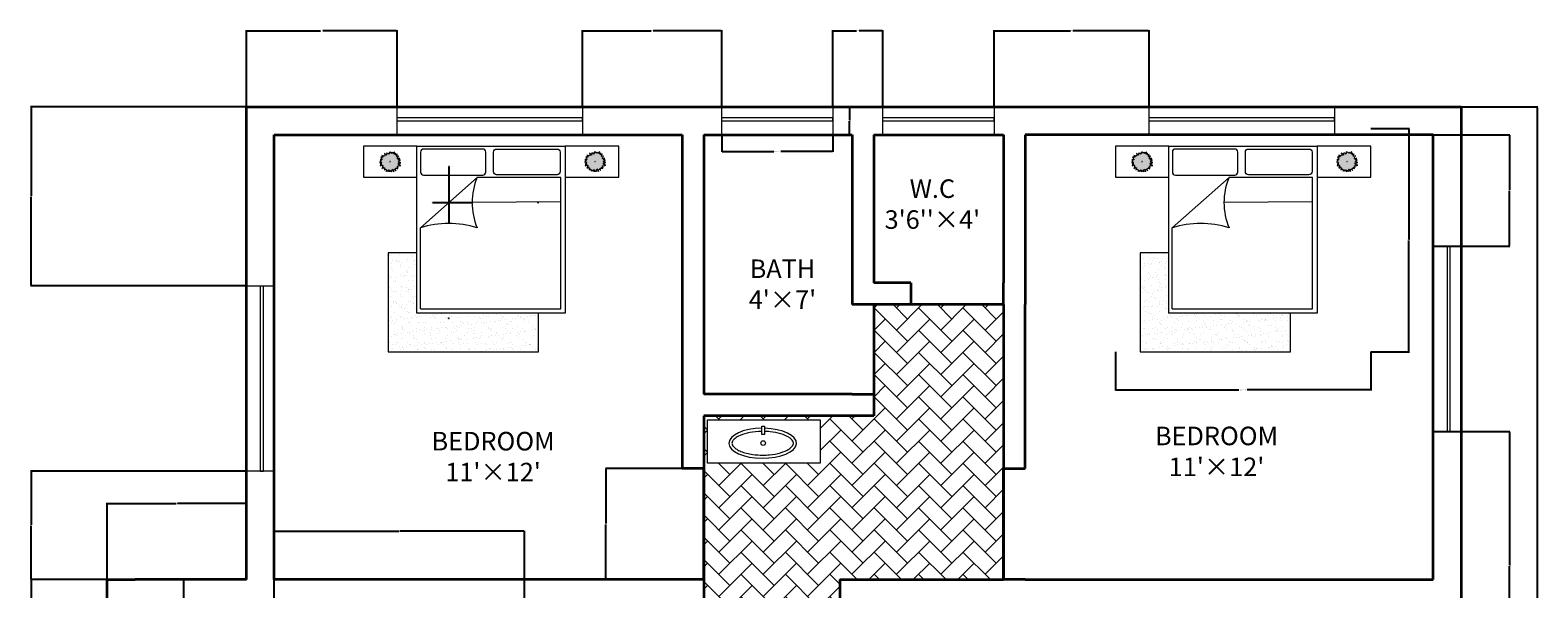
# Model space of a CAD drawing. Units: inches. Extents: x 1315 to 1802, y 1702 to 2202.
# Tile 4 of 4: x 1315 to 1802, y 2021 to 2202. Entities that reach past the tile are written whole.
import ezdxf

# ---------------------------------------------------------------- set-up
doc = ezdxf.new("R2010")
doc.units = ezdxf.units.IN
for name, color, linetype, lineweight in [('A-ANNO-DIMS', 2, 'Continuous', 18), ('A-AREA-IDEN', 3, 'Continuous', 18), ('A-FLOR-FIXT', 30, 'Continuous', 18), ('A-FLOR-PATT', 254, 'Continuous', 13), ('A-FURN', 8, 'Continuous', 18), ('A-GLAZ', 4, 'Continuous', 18), ('A-WALL', 7, 'Continuous', 35)]:
    doc.layers.add(name, color=color, linetype=linetype, lineweight=lineweight)
doc.styles.get("Standard").update_dxf_attribs({"font": 'times.ttf'})
doc.dimstyles.get("Standard").update_dxf_attribs({"dimtxt": 0.18, "dimasz": 0.18, "dimexe": 0.18, "dimexo": 0.0625, "dimgap": 0.09, "dimtad": 0, "dimtih": 1, "dimtoh": 1, "dimdec": 4, "dimzin": 0, "dimdsep": 46, "dimtxsty": 'Standard', "dimcen": 0.09, "dimadec": 0, "dimazin": 0, "dimtfac": 1, "dimtdec": 4, "dimtofl": 0, "dimtmove": 0, "dimatfit": 3, "dimfxl": 1, "dimtolj": 1, "dimtzin": 0, "dimarcsym": 0})

# ---------------------------------------------------------------- blocks, each defined once
blk = doc.blocks.new('*U2')
for points in [[(0, 60.64), (-3.051, 56.238), (-4.196, 52.815), (-5.34, 47.925), (-6.103, 45.969), (-11.062, 50.859), (-18.691, 52.326), (-20.98, 47.436), (-20.217, 43.524), (-20.598, 39.611), (-25.939, 43.035), (-27.846, 49.392), (-33.186, 52.326), (-30.516, 47.436), (-31.279, 43.035), (-30.135, 38.144), (-33.568, 35.21), (-40.815, 36.677), (-49.208, 38.144), (-46.919, 36.677), (-42.341, 31.787), (-42.341, 28.364), (-46.537, 27.386), (-55.692, 27.386), (-49.97, 22.006), (-54.548, 21.028), (-46.156, 14.671), (-51.496, 11.248), (-59.888, 11.248), (-55.692, 8.803), (-53.785, 5.38), (-57.218, 3.423), (-60.651, -1.467), (-61.033, -4.89), (-59.125, -3.423), (-54.548, -1.467), (-51.496, -4.401), (-53.022, -10.269), (-59.125, -15.16), (-49.208, -13.204), (-58.362, -24.451), (-48.445, -21.028), (-43.486, -22.495), (-43.104, -25.918), (-47.3, -31.298), (-43.104, -30.32), (-48.445, -39.611), (-38.527, -31.787), (-40.815, -36.188), (-32.423, -37.166), (-33.568, -43.523), (-35.475, -49.392), (-28.609, -44.99), (-23.65, -46.457), (-22.124, -51.837), (-21.743, -57.705), (-19.073, -52.326), (-15.639, -51.837), (-12.588, -58.683), (-11.062, -54.771), (-6.866, -49.392), (-6.866, -53.304), (-4.959, -48.414), (-1.907, -61.617), (-1.144, -51.348), (4.578, -59.172), (5.341, -54.282), (9.918, -56.727), (12.207, -60.639), (12.97, -47.925), (14.877, -44.501), (17.547, -47.436), (19.455, -52.815), (22.888, -60.639), (21.743, -49.392), (23.65, -46.457), (29.754, -47.925), (35.094, -52.326), (37.001, -53.793), (33.187, -46.457), (32.042, -41.567), (35.094, -39.122), (43.868, -40.589), (47.682, -42.056), (43.105, -36.188), (43.105, -33.743), (46.538, -31.298), (50.352, -32.765), (46.919, -26.407), (55.693, -22.495), (60.652, -22.984), (66.374, -22.006), (59.889, -20.05), (54.167, -18.094), (51.878, -15.649), (49.589, -12.225), (51.497, -10.269), (57.981, -9.78), (63.322, -7.335), (64.466, -2.934)], [(64.848, -2.934), (59.507, -5.379), (56.456, -4.401), (51.878, -2.445), (52.26, 0.978), (55.311, 3.912), (59.889, 5.869), (62.94, 11.248), (58.363, 10.27), (54.548, 10.27), (51.115, 11.248), (53.785, 15.649), (57.981, 18.094), (60.652, 19.561), (56.074, 19.561), (51.115, 17.605), (46.538, 19.072), (46.156, 22.496), (49.589, 27.386), (52.26, 34.721), (49.589, 33.743), (44.249, 30.32), (41.197, 32.276), (41.579, 37.655), (43.868, 42.546), (43.105, 46.947), (40.053, 44.013), (36.238, 40.589), (33.568, 42.057), (33.95, 45.969), (35.476, 52.815), (31.28, 49.392), (26.702, 46.947), (28.228, 50.859), (28.609, 61.129), (24.795, 54.282), (18.692, 50.859), (17.929, 57.706), (12.97, 50.859), (7.248, 57.706), (5.341, 53.304), (0, 60.64)]]:
    blk.add_lwpolyline(points)
blk.add_lwpolyline([(0.382, 1.956), (0, 0), (1.907, 0.489), (2.289, 1.467)], close=True)
blk = doc.blocks.new('BEEDDDDDD')
h = blk.add_hatch(color=256)
h.dxf.hatch_style = 1
h.paths.add_polyline_path([(1431.03, 2159.45), (1431.05, 2159.56), (1431.15, 2159.53), (1431.13, 2159.48)], flags=16)
h.paths.add_polyline_path([(1428.71, 2158.25), (1428.73, 2158.07), (1428.51, 2157.78), (1428.73, 2157.84), (1428.45, 2157.34), (1428.98, 2157.76), (1428.85, 2157.52), (1429.3, 2157.47), (1429.24, 2157.13), (1429.14, 2156.82), (1429.51, 2157.05), (1429.77, 2156.98), (1429.85, 2156.69), (1429.87, 2156.38), (1430.01, 2156.66), (1430.2, 2156.69), (1430.36, 2156.32), (1430.44, 2156.53), (1430.66, 2156.82), (1430.66, 2156.61), (1430.77, 2156.87), (1430.93, 2156.17), (1430.97, 2156.72), (1431.28, 2156.3), (1431.32, 2156.56), (1431.56, 2156.43), (1431.68, 2156.22), (1431.72, 2156.9), (1431.82, 2157.08), (1431.97, 2156.92), (1432.07, 2156.64), (1432.25, 2156.22), (1432.19, 2156.82), (1432.29, 2156.98), (1432.62, 2156.9), (1432.9, 2156.66), (1433, 2156.58), (1432.8, 2156.98), (1432.74, 2157.24), (1432.9, 2157.37), (1433.37, 2157.29), (1433.57, 2157.21), (1433.33, 2157.52), (1433.33, 2157.65), (1433.51, 2157.78), (1433.72, 2157.71), (1433.53, 2158.05), (1434, 2158.25), (1434.26, 2158.23), (1434.57, 2158.28), (1434.22, 2158.38), (1433.92, 2158.49), (1433.8, 2158.62), (1433.67, 2158.8), (1433.78, 2158.91), (1434.12, 2158.93), (1434.41, 2159.06), (1434.47, 2159.29), (1434.2, 2159.17), (1434.04, 2159.22), (1433.8, 2159.32), (1433.82, 2159.51), (1433.98, 2159.66), (1434.22, 2159.77), (1434.39, 2160.05), (1434.14, 2160), (1433.94, 2160), (1433.76, 2160.05), (1433.9, 2160.29), (1434.12, 2160.42), (1434.26, 2160.5), (1434.02, 2160.5), (1433.76, 2160.39), (1433.51, 2160.47), (1433.49, 2160.65), (1433.67, 2160.91), (1433.82, 2161.3), (1433.67, 2161.25), (1433.39, 2161.07), (1433.23, 2161.17), (1433.25, 2161.46), (1433.37, 2161.72), (1433.33, 2161.96), (1433.17, 2161.8), (1432.96, 2161.62), (1432.82, 2161.7), (1432.84, 2161.9), (1432.92, 2162.27), (1432.7, 2162.09), (1432.45, 2161.96), (1432.54, 2162.16), (1432.56, 2162.71), (1432.35, 2162.35), (1432.03, 2162.16), (1431.99, 2162.53), (1431.72, 2162.16), (1431.42, 2162.53), (1431.32, 2162.3), (1431.03, 2162.69), (1430.87, 2162.45), (1430.81, 2162.27), (1430.72, 2161.89), (1430.44, 2162.16), (1430.03, 2162.24), (1429.91, 2161.98), (1429.95, 2161.77), (1429.93, 2161.56), (1429.65, 2161.75), (1429.55, 2162.09), (1429.26, 2162.24), (1429.4, 2161.98), (1429.36, 2161.75), (1429.42, 2161.49), (1429.24, 2161.33), (1428.85, 2161.41), (1428.41, 2161.49), (1428.53, 2161.41), (1428.77, 2161.15), (1428.77, 2160.97), (1428.55, 2160.91), (1428.06, 2160.91), (1428.37, 2160.63), (1428.12, 2160.57), (1428.57, 2160.24), (1428.29, 2160.05), (1427.84, 2160.05), (1428.06, 2159.92), (1428.16, 2159.74), (1427.98, 2159.64), (1427.8, 2159.37), (1427.78, 2159.19), (1427.88, 2159.27), (1428.12, 2159.37), (1428.29, 2159.22), (1428.2, 2158.91), (1427.88, 2158.64), (1428.41, 2158.75), (1427.92, 2158.15), (1428.45, 2158.33)])
h = blk.add_hatch(color=256)
h.dxf.hatch_style = 1
h.paths.add_polyline_path([(1500.43, 2158.99), (1500.72, 2159.12), (1500.78, 2159.35), (1500.52, 2159.23), (1500.35, 2159.28), (1500.11, 2159.38), (1500.13, 2159.57), (1500.29, 2159.72), (1500.54, 2159.83), (1500.7, 2160.11), (1500.45, 2160.06), (1500.25, 2160.06), (1500.07, 2160.11), (1500.21, 2160.35), (1500.43, 2160.48), (1500.58, 2160.56), (1500.33, 2160.56), (1500.07, 2160.45), (1499.82, 2160.53), (1499.8, 2160.71), (1499.99, 2160.97), (1500.13, 2161.37), (1499.99, 2161.31), (1499.7, 2161.13), (1499.54, 2161.24), (1499.56, 2161.52), (1499.68, 2161.78), (1499.64, 2162.02), (1499.48, 2161.86), (1499.28, 2161.68), (1499.13, 2161.76), (1499.15, 2161.97), (1499.23, 2162.33), (1499.01, 2162.15), (1498.77, 2162.02), (1498.85, 2162.23), (1498.87, 2162.77), (1498.67, 2162.41), (1498.34, 2162.23), (1498.3, 2162.59), (1498.03, 2162.23), (1497.73, 2162.59), (1497.63, 2162.36), (1497.34, 2162.75), (1497.18, 2162.51), (1497.12, 2162.33), (1497.06, 2162.07), (1497.02, 2161.97), (1496.75, 2162.23), (1496.35, 2162.3), (1496.22, 2162.04), (1496.27, 2161.84), (1496.24, 2161.63), (1495.96, 2161.81), (1495.86, 2162.15), (1495.57, 2162.3), (1495.72, 2162.04), (1495.68, 2161.81), (1495.74, 2161.55), (1495.55, 2161.39), (1495.17, 2161.47), (1494.72, 2161.55), (1494.84, 2161.47), (1495.09, 2161.21), (1495.09, 2161.03), (1494.86, 2160.97), (1494.37, 2160.97), (1494.68, 2160.69), (1494.43, 2160.64), (1494.88, 2160.3), (1494.6, 2160.11), (1494.15, 2160.11), (1494.37, 2159.98), (1494.48, 2159.8), (1494.29, 2159.7), (1494.11, 2159.44), (1494.09, 2159.25), (1494.19, 2159.33), (1494.43, 2159.44), (1494.6, 2159.28), (1494.52, 2158.97), (1494.19, 2158.71), (1494.72, 2158.81), (1494.23, 2158.21), (1494.76, 2158.39), (1495.02, 2158.32), (1495.04, 2158.13), (1494.82, 2157.85), (1495.04, 2157.9), (1494.76, 2157.4), (1495.29, 2157.82), (1495.17, 2157.59), (1495.61, 2157.53), (1495.55, 2157.19), (1495.45, 2156.88), (1495.82, 2157.12), (1496.08, 2157.04), (1496.16, 2156.75), (1496.18, 2156.44), (1496.33, 2156.72), (1496.51, 2156.75), (1496.67, 2156.39), (1496.75, 2156.59), (1496.98, 2156.88), (1496.98, 2156.67), (1497.08, 2156.93), (1497.24, 2156.23), (1497.28, 2156.78), (1497.59, 2156.36), (1497.63, 2156.62), (1497.87, 2156.49), (1497.99, 2156.28), (1498.03, 2156.96), (1498.14, 2157.14), (1498.28, 2156.99), (1498.38, 2156.7), (1498.56, 2156.28), (1498.5, 2156.88), (1498.6, 2157.04), (1498.93, 2156.96), (1499.21, 2156.72), (1499.32, 2156.65), (1499.11, 2157.04), (1499.05, 2157.3), (1499.21, 2157.43), (1499.68, 2157.35), (1499.89, 2157.27), (1499.64, 2157.59), (1499.64, 2157.72), (1499.82, 2157.85), (1500.03, 2157.77), (1499.84, 2158.11), (1500.31, 2158.32), (1500.58, 2158.29), (1500.88, 2158.34), (1500.54, 2158.45), (1500.23, 2158.55), (1500.11, 2158.68), (1499.99, 2158.86), (1500.09, 2158.97)])
h.paths.add_polyline_path([(1497.34, 2159.51), (1497.36, 2159.62), (1497.47, 2159.59), (1497.44, 2159.54)], flags=16)
h = blk.add_hatch()
h.set_pattern_fill('AR-SAND', color=256, scale=0.07)
h.paths.add_polyline_path([(1479.13, 2098), (1479.13, 2110.5), (1439.77, 2110.5), (1439.77, 2129.95), (1430.49, 2129.95), (1430.49, 2098)])
for p, q in [((1439.77, 2164.5), (1422.47, 2164.5)), ((1422.47, 2164.5), (1422.47, 2154.5)), ((1439.77, 2164.5), (1487.77, 2164.5)), ((1439.77, 2110.5), (1439.77, 2164.5)), ((1439.77, 2154.5), (1439.77, 2164.5)), ((1487.77, 2164.5), (1487.77, 2110.5)), ((1505.08, 2164.5), (1487.77, 2164.5)), ((1487.77, 2164.5), (1487.77, 2154.5)), ((1505.08, 2154.5), (1505.08, 2164.5)), ((1422.47, 2154.5), (1439.77, 2154.5)), ((1440.88, 2138.11), (1459.24, 2154.43)), ((1486.29, 2154.43), (1459.24, 2154.43)), ((1486.29, 2111.9), (1486.29, 2154.43)), ((1487.77, 2154.5), (1505.08, 2154.5)), ((1486.29, 2146.5), (1457.62, 2146.27)), ((1440.88, 2111.9), (1440.88, 2138.11)), ((1439.77, 2129.95), (1430.49, 2129.95)), ((1430.49, 2129.95), (1430.49, 2098)), ((1487.77, 2110.5), (1439.77, 2110.5)), ((1440.88, 2111.9), (1486.29, 2111.9)), ((1479.13, 2098), (1479.13, 2110.5)), ((1430.49, 2098), (1479.13, 2098))]:
    blk.add_line(p, q)
for points in [[(1461.08, 2163.58), (1441.91, 2163.58, 0.414214), (1440.91, 2162.58), (1440.91, 2156.15, 0.414214), (1441.91, 2155.15), (1461.08, 2155.15, 0.414214), (1462.08, 2156.15), (1462.08, 2162.58, 0.414214)], [(1485.11, 2155.25), (1465.55, 2155.25, -0.414214), (1464.55, 2156.25), (1464.55, 2162.58, -0.414214), (1465.55, 2163.58), (1485.11, 2163.58, -0.414214), (1486.11, 2162.58), (1486.11, 2156.25, -0.414214)]]:
    blk.add_lwpolyline(points, format="xyb", close=True)
for centre, radius, start, end in [((1479, 2146.27), 21.38, 157.5543, 202.4457), ((1450.06, 2108.85), 30.67, 72.5775, 107.4225)]:
    blk.add_arc(centre, radius, start, end)
at = {"xscale": 0.0533167339335912, "yscale": 0.0533167339335912, "zscale": 0.0533167339335912}
for p in [(1431.03, 2159.45), (1497.34, 2159.51)]:
    blk.add_blockref('*U2', p, dxfattribs=at)
blk = doc.blocks.new('SEFVFT')
for p, q in [((1768.59, 1985.26), (1777.59, 1985.26)), ((1768.59, 1925.26), (1768.59, 1985.26)), ((1768.59, 1985.26), (1773.09, 1985.26)), ((1773.09, 1985.26), (1773.09, 1925.26)), ((1774.09, 1925.26), (1774.09, 1985.26)), ((1777.59, 1985.26), (1777.59, 1925.26)), ((1777.59, 1925.26), (1768.59, 1925.26)), ((1773.09, 1925.26), (1774.09, 1925.26))]:
    blk.add_line(p, q)
blk = doc.blocks.new('WIN-36IN')
for p, q in [((0, 0), (0, 9)), ((0, 9), (36, 9)), ((36, 5.5), (0, 5.5)), ((36, 9), (36, 0)), ((36, 4.5), (36, 5.5)), ((0, 0), (0, 4.5)), ((0, 4.5), (36, 4.5)), ((36, 0), (0, 0))]:
    blk.add_line(p, q)
blk = doc.blocks.new('*D14')
at = {"layer": 'A-ANNO-DIMS', "color": 0, "lineweight": -2, "transparency": 16777216}
for p, q in [((1538.38, 2168.18), (1538.38, 2162.66)), ((1574.38, 2168.18), (1574.38, 2162.66)), ((1538.56, 2162.84), (1555.24, 2162.84)), ((1574.2, 2162.84), (1557.53, 2162.84))]:
    blk.add_line(p, q, dxfattribs=at)
at = {"layer": 'A-ANNO-DIMS', "color": 0, "transparency": 16777216}
for points in [[(1538.56, 2162.87), (1538.56, 2162.81), (1538.38, 2162.84)], [(1574.2, 2162.87), (1574.2, 2162.81), (1574.38, 2162.84)]]:
    blk.add_solid(points, dxfattribs=at)
at = {"layer": 'Defpoints', "color": 0, "transparency": 16777216}
for p in [(1538.38, 2168.24), (1574.38, 2168.24), (1574.38, 2162.84)]:
    blk.add_point(p, dxfattribs=at)
at = {"layer": 'A-ANNO-DIMS', "color": 0, "transparency": 16777216, "insert": (1556.38, 2162.84), "char_height": 0.18, "attachment_point": 5}
blk.add_mtext('\\A1;WINDOW 36 TYP.', dxfattribs=at)
blk = doc.blocks.new('*D15')
at = {"layer": 'A-ANNO-DIMS', "color": 0, "lineweight": -2, "transparency": 16777216}
for p, q in [((1574.45, 2177.24), (1579.96, 2177.24)), ((1579.78, 2177.06), (1579.78, 2172.92)), ((1579.78, 2168.42), (1579.78, 2172.56)), ((1574.45, 2168.24), (1579.96, 2168.24))]:
    blk.add_line(p, q, dxfattribs=at)
at = {"layer": 'A-ANNO-DIMS', "color": 0, "transparency": 16777216}
for points in [[(1579.75, 2177.06), (1579.81, 2177.06), (1579.78, 2177.24)], [(1579.75, 2168.42), (1579.81, 2168.42), (1579.78, 2168.24)]]:
    blk.add_solid(points, dxfattribs=at)
at = {"layer": 'Defpoints', "color": 0, "transparency": 16777216}
for p in [(1574.38, 2177.24), (1579.78, 2177.24), (1574.38, 2168.24)]:
    blk.add_point(p, dxfattribs=at)
at = {"layer": 'A-ANNO-DIMS', "color": 0, "transparency": 16777216, "insert": (1579.78, 2172.74), "char_height": 0.18, "attachment_point": 5}
blk.add_mtext('\\A1;9 TYP.', dxfattribs=at)
blk = doc.blocks.new('*D16')
at = {"layer": 'A-ANNO-DIMS', "color": 0, "lineweight": -2, "transparency": 16777216}
for p, q in [((1665.75, 2097.94), (1665.75, 2085.43)), ((1748.36, 2097.94), (1748.36, 2085.43)), ((1665.93, 2085.61), (1705.74, 2085.61)), ((1748.18, 2085.61), (1708.36, 2085.61))]:
    blk.add_line(p, q, dxfattribs=at)
at = {"layer": 'A-ANNO-DIMS', "color": 0, "transparency": 16777216}
for points in [[(1665.93, 2085.64), (1665.93, 2085.58), (1665.75, 2085.61)], [(1748.18, 2085.64), (1748.18, 2085.58), (1748.36, 2085.61)]]:
    blk.add_solid(points, dxfattribs=at)
at = {"layer": 'Defpoints', "color": 0, "transparency": 16777216}
for p in [(1665.75, 2098), (1748.36, 2098), (1748.36, 2085.61)]:
    blk.add_point(p, dxfattribs=at)
at = {"layer": 'A-ANNO-DIMS', "color": 0, "transparency": 16777216, "insert": (1707.05, 2085.61), "char_height": 0.18, "attachment_point": 5}
blk.add_mtext('\\A1;BED GROUP 83 TYP.', dxfattribs=at)
blk = doc.blocks.new('*D17')
at = {"layer": 'A-ANNO-DIMS', "color": 0, "lineweight": -2, "transparency": 16777216}
for p, q in [((1748.42, 2170.24), (1760.93, 2170.24)), ((1760.75, 2170.06), (1760.75, 2134.3)), ((1760.75, 2098.18), (1760.75, 2133.94)), ((1748.42, 2098), (1760.93, 2098))]:
    blk.add_line(p, q, dxfattribs=at)
at = {"layer": 'A-ANNO-DIMS', "color": 0, "transparency": 16777216}
for points in [[(1760.72, 2170.06), (1760.78, 2170.06), (1760.75, 2170.24)], [(1760.72, 2098.18), (1760.78, 2098.18), (1760.75, 2098)]]:
    blk.add_solid(points, dxfattribs=at)
at = {"layer": 'Defpoints', "color": 0, "transparency": 16777216}
for p in [(1748.36, 2170.24), (1760.75, 2170.24), (1748.36, 2098)]:
    blk.add_point(p, dxfattribs=at)
at = {"layer": 'A-ANNO-DIMS', "color": 0, "transparency": 16777216, "insert": (1760.75, 2134.12), "char_height": 0.18, "attachment_point": 5}
blk.add_mtext('\\A1;72 TYP.', dxfattribs=at)
blk = doc.blocks.new('*D29')
at = {"layer": 'A-ANNO-DIMS', "color": 0, "lineweight": -2, "transparency": 16777216}
for p, q in [((1777.65, 2177.24), (1802.42, 2177.24)), ((1802.24, 2177.06), (1802.24, 1952.42)), ((1802.24, 1727.42), (1802.24, 1952.06)), ((1645.65, 1727.24), (1802.42, 1727.24))]:
    blk.add_line(p, q, dxfattribs=at)
at = {"layer": 'A-ANNO-DIMS', "color": 0, "transparency": 16777216}
for points in [[(1802.21, 2177.06), (1802.27, 2177.06), (1802.24, 2177.24)], [(1802.21, 1727.42), (1802.27, 1727.42), (1802.24, 1727.24)]]:
    blk.add_solid(points, dxfattribs=at)
at = {"layer": 'Defpoints', "color": 0, "transparency": 16777216}
for p in [(1777.59, 2177.24), (1802.24, 2177.24), (1645.59, 1727.24)]:
    blk.add_point(p, dxfattribs=at)
at = {"layer": 'A-ANNO-DIMS', "color": 0, "transparency": 16777216, "insert": (1802.24, 1952.24), "char_height": 0.18, "attachment_point": 5}
blk.add_mtext('\\A1;450', dxfattribs=at)
blk = doc.blocks.new('*D30')
at = {"layer": 'A-ANNO-DIMS', "color": 0, "lineweight": -2, "transparency": 16777216}
for p, q in [((1339.59, 2024.3), (1339.59, 2049.07)), ((1339.77, 2048.89), (1361.88, 2048.89)), ((1384.41, 2048.89), (1362.3, 2048.89)), ((1384.59, 2024.3), (1384.59, 2049.07))]:
    blk.add_line(p, q, dxfattribs=at)
at = {"layer": 'A-ANNO-DIMS', "color": 0, "transparency": 16777216}
for points in [[(1339.77, 2048.92), (1339.77, 2048.86), (1339.59, 2048.89)], [(1384.41, 2048.92), (1384.41, 2048.86), (1384.59, 2048.89)]]:
    blk.add_solid(points, dxfattribs=at)
at = {"layer": 'Defpoints', "color": 0, "transparency": 16777216}
for p in [(1384.59, 2048.89), (1339.59, 2024.24), (1384.59, 2024.24)]:
    blk.add_point(p, dxfattribs=at)
at = {"layer": 'A-ANNO-DIMS', "color": 0, "transparency": 16777216, "insert": (1362.09, 2048.89), "char_height": 0.18, "attachment_point": 5}
blk.add_mtext('\\A1;45', dxfattribs=at)
blk = doc.blocks.new('*D31')
at = {"layer": 'A-ANNO-DIMS', "color": 0, "lineweight": -2, "transparency": 16777216}
for p, q in [((1384.59, 2177.3), (1384.59, 2202.07)), ((1384.77, 2201.89), (1408.6, 2201.89)), ((1433.2, 2201.89), (1409.36, 2201.89)), ((1433.38, 2177.3), (1433.38, 2202.07))]:
    blk.add_line(p, q, dxfattribs=at)
at = {"layer": 'A-ANNO-DIMS', "color": 0, "transparency": 16777216}
for points in [[(1384.77, 2201.92), (1384.77, 2201.86), (1384.59, 2201.89)], [(1433.2, 2201.92), (1433.2, 2201.86), (1433.38, 2201.89)]]:
    blk.add_solid(points, dxfattribs=at)
at = {"layer": 'Defpoints', "color": 0, "transparency": 16777216}
for p in [(1433.38, 2201.89), (1384.59, 2177.24), (1433.38, 2177.24)]:
    blk.add_point(p, dxfattribs=at)
at = {"layer": 'A-ANNO-DIMS', "color": 0, "transparency": 16777216, "insert": (1408.98, 2201.89), "char_height": 0.18, "attachment_point": 5}
blk.add_mtext('\\A1;48.79', dxfattribs=at)
blk = doc.blocks.new('*D32')
at = {"layer": 'A-ANNO-DIMS', "color": 0, "lineweight": -2, "transparency": 16777216}
for p, q in [((1493.38, 2177.3), (1493.38, 2202.07)), ((1493.56, 2201.89), (1515.51, 2201.89)), ((1538.2, 2201.89), (1516.25, 2201.89)), ((1538.38, 2177.3), (1538.38, 2202.07))]:
    blk.add_line(p, q, dxfattribs=at)
at = {"layer": 'A-ANNO-DIMS', "color": 0, "transparency": 16777216}
for points in [[(1493.56, 2201.92), (1493.56, 2201.86), (1493.38, 2201.89)], [(1538.2, 2201.92), (1538.2, 2201.86), (1538.38, 2201.89)]]:
    blk.add_solid(points, dxfattribs=at)
at = {"layer": 'Defpoints', "color": 0, "transparency": 16777216}
for p in [(1538.38, 2201.89), (1493.38, 2177.24), (1538.38, 2177.24)]:
    blk.add_point(p, dxfattribs=at)
at = {"layer": 'A-ANNO-DIMS', "color": 0, "transparency": 16777216, "insert": (1515.88, 2201.89), "char_height": 0.18, "attachment_point": 5}
blk.add_mtext('\\A1;45.01', dxfattribs=at)
blk = doc.blocks.new('*D33')
at = {"layer": 'A-ANNO-DIMS', "color": 0, "lineweight": -2, "transparency": 16777216}
for p, q in [((1574.38, 2177.3), (1574.38, 2202.07)), ((1574.56, 2201.89), (1582.01, 2201.89)), ((1590.33, 2201.89), (1582.88, 2201.89)), ((1590.51, 2177.3), (1590.51, 2202.07))]:
    blk.add_line(p, q, dxfattribs=at)
at = {"layer": 'A-ANNO-DIMS', "color": 0, "transparency": 16777216}
for points in [[(1574.56, 2201.92), (1574.56, 2201.86), (1574.38, 2201.89)], [(1590.33, 2201.92), (1590.33, 2201.86), (1590.51, 2201.89)]]:
    blk.add_solid(points, dxfattribs=at)
at = {"layer": 'Defpoints', "color": 0, "transparency": 16777216}
for p in [(1590.51, 2201.89), (1574.38, 2177.24), (1590.51, 2177.24)]:
    blk.add_point(p, dxfattribs=at)
at = {"layer": 'A-ANNO-DIMS', "color": 0, "transparency": 16777216, "insert": (1582.45, 2201.89), "char_height": 0.18, "attachment_point": 5}
blk.add_mtext('\\A1;16.127', dxfattribs=at)
blk = doc.blocks.new('*D34')
at = {"layer": 'A-ANNO-DIMS', "color": 0, "lineweight": -2, "transparency": 16777216}
for p, q in [((1626.51, 2177.3), (1626.51, 2202.07)), ((1626.69, 2201.89), (1651.21, 2201.89)), ((1676.48, 2201.89), (1651.96, 2201.89)), ((1676.66, 2177.3), (1676.66, 2202.07))]:
    blk.add_line(p, q, dxfattribs=at)
at = {"layer": 'A-ANNO-DIMS', "color": 0, "transparency": 16777216}
for points in [[(1626.69, 2201.92), (1626.69, 2201.86), (1626.51, 2201.89)], [(1676.48, 2201.92), (1676.48, 2201.86), (1676.66, 2201.89)]]:
    blk.add_solid(points, dxfattribs=at)
at = {"layer": 'Defpoints', "color": 0, "transparency": 16777216}
for p in [(1676.66, 2201.89), (1626.51, 2177.24), (1676.66, 2177.24)]:
    blk.add_point(p, dxfattribs=at)
at = {"layer": 'A-ANNO-DIMS', "color": 0, "transparency": 16777216, "insert": (1651.58, 2201.89), "char_height": 0.18, "attachment_point": 5}
blk.add_mtext('\\A1;50.15', dxfattribs=at)
blk = doc.blocks.new('*D35')
at = {"layer": 'A-ANNO-DIMS', "color": 0, "lineweight": -2, "transparency": 16777216}
for p, q in [((1384.53, 2177.24), (1314.76, 2177.24)), ((1314.94, 2177.06), (1314.94, 2148.46)), ((1314.94, 2119.5), (1314.94, 2148.1)), ((1384.53, 2119.32), (1314.76, 2119.32))]:
    blk.add_line(p, q, dxfattribs=at)
at = {"layer": 'A-ANNO-DIMS', "color": 0, "transparency": 16777216}
for points in [[(1314.91, 2177.06), (1314.97, 2177.06), (1314.94, 2177.24)], [(1314.91, 2119.5), (1314.97, 2119.5), (1314.94, 2119.32)]]:
    blk.add_solid(points, dxfattribs=at)
at = {"layer": 'Defpoints', "color": 0, "transparency": 16777216}
for p in [(1384.59, 2177.24), (1314.94, 2119.32), (1384.59, 2119.32)]:
    blk.add_point(p, dxfattribs=at)
at = {"layer": 'A-ANNO-DIMS', "color": 0, "transparency": 16777216, "insert": (1314.94, 2148.28), "char_height": 0.18, "attachment_point": 5}
blk.add_mtext('\\A1;57.92', dxfattribs=at)
blk = doc.blocks.new('*D36')
at = {"layer": 'A-ANNO-DIMS', "color": 0, "lineweight": -2, "transparency": 16777216}
for p, q in [((1384.53, 2059.32), (1314.76, 2059.32)), ((1314.94, 2059.14), (1314.94, 2041.96)), ((1314.94, 2024.42), (1314.94, 2041.6)), ((1384.53, 2024.24), (1314.76, 2024.24))]:
    blk.add_line(p, q, dxfattribs=at)
at = {"layer": 'A-ANNO-DIMS', "color": 0, "transparency": 16777216}
for points in [[(1314.91, 2059.14), (1314.97, 2059.14), (1314.94, 2059.32)], [(1314.91, 2024.42), (1314.97, 2024.42), (1314.94, 2024.24)]]:
    blk.add_solid(points, dxfattribs=at)
at = {"layer": 'Defpoints', "color": 0, "transparency": 16777216}
for p in [(1384.59, 2059.32), (1314.94, 2024.24), (1384.59, 2024.24)]:
    blk.add_point(p, dxfattribs=at)
at = {"layer": 'A-ANNO-DIMS', "color": 0, "transparency": 16777216, "insert": (1314.94, 2041.78), "char_height": 0.18, "attachment_point": 5}
blk.add_mtext('\\A1;35.08', dxfattribs=at)
blk = doc.blocks.new('*D37')
at = {"layer": 'A-ANNO-DIMS', "color": 0, "lineweight": -2, "transparency": 16777216}
for p, q in [((1339.53, 2024.24), (1314.76, 2024.24)), ((1314.94, 2024.06), (1314.94, 1977.92)), ((1314.94, 1931.42), (1314.94, 1977.56)), ((1339.53, 1931.24), (1314.76, 1931.24))]:
    blk.add_line(p, q, dxfattribs=at)
at = {"layer": 'A-ANNO-DIMS', "color": 0, "transparency": 16777216}
for points in [[(1314.91, 2024.06), (1314.97, 2024.06), (1314.94, 2024.24)], [(1314.91, 1931.42), (1314.97, 1931.42), (1314.94, 1931.24)]]:
    blk.add_solid(points, dxfattribs=at)
at = {"layer": 'Defpoints', "color": 0, "transparency": 16777216}
for p in [(1339.59, 2024.24), (1314.94, 1931.24), (1339.59, 1931.24)]:
    blk.add_point(p, dxfattribs=at)
at = {"layer": 'A-ANNO-DIMS', "color": 0, "transparency": 16777216, "insert": (1314.94, 1977.74), "char_height": 0.18, "attachment_point": 5}
blk.add_mtext('\\A1;93', dxfattribs=at)
blk = doc.blocks.new('*D38')
at = {"layer": 'A-ANNO-DIMS', "color": 0, "lineweight": -2, "transparency": 16777216}
for p, q in [((1339.65, 2024.24), (1364.42, 2024.24)), ((1364.24, 2024.06), (1364.24, 2015.88)), ((1364.24, 2007.33), (1364.24, 2015.51)), ((1339.65, 2007.15), (1364.42, 2007.15))]:
    blk.add_line(p, q, dxfattribs=at)
at = {"layer": 'A-ANNO-DIMS', "color": 0, "transparency": 16777216}
for points in [[(1364.21, 2024.06), (1364.27, 2024.06), (1364.24, 2024.24)], [(1364.21, 2007.33), (1364.27, 2007.33), (1364.24, 2007.15)]]:
    blk.add_solid(points, dxfattribs=at)
at = {"layer": 'Defpoints', "color": 0, "transparency": 16777216}
for p in [(1339.59, 2024.24), (1339.59, 2007.15), (1364.24, 2007.15)]:
    blk.add_point(p, dxfattribs=at)
at = {"layer": 'A-ANNO-DIMS', "color": 0, "transparency": 16777216, "insert": (1364.24, 2015.69), "char_height": 0.18, "attachment_point": 5}
blk.add_mtext('\\A1;17.095', dxfattribs=at)
blk = doc.blocks.new('*D41')
at = {"layer": 'A-ANNO-DIMS', "color": 0, "lineweight": -2, "transparency": 16777216}
for p, q in [((1768.65, 2168.24), (1793.42, 2168.24)), ((1793.24, 2168.06), (1793.24, 2150.4)), ((1793.24, 2132.37), (1793.24, 2150.04)), ((1768.65, 2132.19), (1793.42, 2132.19))]:
    blk.add_line(p, q, dxfattribs=at)
at = {"layer": 'A-ANNO-DIMS', "color": 0, "transparency": 16777216}
for points in [[(1793.21, 2168.06), (1793.27, 2168.06), (1793.24, 2168.24)], [(1793.21, 2132.37), (1793.27, 2132.37), (1793.24, 2132.19)]]:
    blk.add_solid(points, dxfattribs=at)
at = {"layer": 'Defpoints', "color": 0, "transparency": 16777216}
for p in [(1768.59, 2168.24), (1768.59, 2132.19), (1793.24, 2132.19)]:
    blk.add_point(p, dxfattribs=at)
at = {"layer": 'A-ANNO-DIMS', "color": 0, "transparency": 16777216, "insert": (1793.24, 2150.22), "char_height": 0.18, "attachment_point": 5}
blk.add_mtext('\\A1;36.05', dxfattribs=at)
blk = doc.blocks.new('*D42')
at = {"layer": 'A-ANNO-DIMS', "color": 0, "lineweight": -2, "transparency": 16777216}
for p, q in [((1768.65, 2072.19), (1793.42, 2072.19)), ((1793.24, 2072.01), (1793.24, 2028.91)), ((1793.24, 1985.44), (1793.24, 2028.54)), ((1768.65, 1985.26), (1793.42, 1985.26))]:
    blk.add_line(p, q, dxfattribs=at)
at = {"layer": 'A-ANNO-DIMS', "color": 0, "transparency": 16777216}
for points in [[(1793.21, 2072.01), (1793.27, 2072.01), (1793.24, 2072.19)], [(1793.21, 1985.44), (1793.27, 1985.44), (1793.24, 1985.26)]]:
    blk.add_solid(points, dxfattribs=at)
at = {"layer": 'Defpoints', "color": 0, "transparency": 16777216}
for p in [(1768.59, 2072.19), (1768.59, 1985.26), (1793.24, 1985.26)]:
    blk.add_point(p, dxfattribs=at)
at = {"layer": 'A-ANNO-DIMS', "color": 0, "transparency": 16777216, "insert": (1793.24, 2028.72), "char_height": 0.18, "attachment_point": 5}
blk.add_mtext('\\A1;86.94', dxfattribs=at)
blk = doc.blocks.new('*D50')
at = {"layer": 'A-ANNO-DIMS', "color": 0, "lineweight": -2, "transparency": 16777216}
for p, q in [((1393.59, 2015.3), (1393.59, 2040.07)), ((1393.77, 2039.89), (1433.89, 2039.89)), ((1474.41, 2039.89), (1434.29, 2039.89)), ((1474.59, 2015.3), (1474.59, 2040.07))]:
    blk.add_line(p, q, dxfattribs=at)
at = {"layer": 'A-ANNO-DIMS', "color": 0, "transparency": 16777216}
for points in [[(1393.77, 2039.92), (1393.77, 2039.86), (1393.59, 2039.89)], [(1474.41, 2039.92), (1474.41, 2039.86), (1474.59, 2039.89)]]:
    blk.add_solid(points, dxfattribs=at)
at = {"layer": 'Defpoints', "color": 0, "transparency": 16777216}
for p in [(1474.59, 2039.89), (1393.59, 2015.24), (1474.59, 2015.24)]:
    blk.add_point(p, dxfattribs=at)
at = {"layer": 'A-ANNO-DIMS', "color": 0, "transparency": 16777216, "insert": (1434.09, 2039.89), "char_height": 0.18, "attachment_point": 5}
blk.add_mtext('\\A1;81', dxfattribs=at)
blk = doc.blocks.new('*D53')
at = {"layer": 'A-ANNO-DIMS', "color": 0, "lineweight": -2, "transparency": 16777216}
for p, q in [((1525.53, 2060.24), (1500.76, 2060.24)), ((1500.94, 2060.06), (1500.94, 2042.42)), ((1500.94, 2024.42), (1500.94, 2042.06)), ((1525.53, 2024.24), (1500.76, 2024.24))]:
    blk.add_line(p, q, dxfattribs=at)
at = {"layer": 'A-ANNO-DIMS', "color": 0, "transparency": 16777216}
for points in [[(1500.91, 2060.06), (1500.97, 2060.06), (1500.94, 2060.24)], [(1500.91, 2024.42), (1500.97, 2024.42), (1500.94, 2024.24)]]:
    blk.add_solid(points, dxfattribs=at)
at = {"layer": 'Defpoints', "color": 0, "transparency": 16777216}
for p in [(1500.94, 2060.24), (1525.59, 2060.24), (1525.59, 2024.24)]:
    blk.add_point(p, dxfattribs=at)
at = {"layer": 'A-ANNO-DIMS', "color": 0, "transparency": 16777216, "insert": (1500.94, 2042.24), "char_height": 0.18, "attachment_point": 5}
blk.add_mtext('\\A1;36', dxfattribs=at)
blk = doc.blocks.new('*D58')
at = {"layer": 'A-ANNO-DIMS', "color": 0, "lineweight": -2, "transparency": 16777216}
for p, q in [((1450.24, 2157.92), (1450.06, 2157.92)), ((1450.06, 2157.92), (1450.06, 2139.7)), ((1449.97, 2108.85), (1450.15, 2108.85)), ((1450.06, 2108.76), (1450.06, 2108.94))]:
    blk.add_line(p, q, dxfattribs=at)
at = {"layer": 'A-ANNO-DIMS', "color": 0, "transparency": 16777216}
blk.add_solid([(1450.03, 2139.7), (1450.09, 2139.7), (1450.06, 2139.52)], dxfattribs=at)
at = {"layer": 'Defpoints', "color": 0, "transparency": 16777216}
for p in [(1450.06, 2139.52), (1450.06, 2108.85)]:
    blk.add_point(p, dxfattribs=at)
at = {"layer": 'A-ANNO-DIMS', "color": 0, "transparency": 16777216, "insert": (1450.91, 2157.92), "char_height": 0.18, "attachment_point": 5}
blk.add_mtext('\\A1;2X R30.67', dxfattribs=at)
blk = doc.blocks.new('*D59')
at = {"layer": 'A-ANNO-DIMS', "color": 0, "lineweight": -2, "transparency": 16777216}
for p, q in [((1444.8, 2146.27), (1457.44, 2146.27)), ((1478.91, 2146.27), (1479.09, 2146.27)), ((1479, 2146.18), (1479, 2146.36))]:
    blk.add_line(p, q, dxfattribs=at)
at = {"layer": 'A-ANNO-DIMS', "color": 0, "transparency": 16777216}
blk.add_solid([(1457.44, 2146.3), (1457.44, 2146.24), (1457.62, 2146.27)], dxfattribs=at)
at = {"layer": 'Defpoints', "color": 0, "transparency": 16777216}
for p in [(1457.62, 2146.27), (1479, 2146.27)]:
    blk.add_point(p, dxfattribs=at)
at = {"layer": 'A-ANNO-DIMS', "color": 0, "transparency": 16777216, "insert": (1444.07, 2146.27), "char_height": 0.18, "attachment_point": 5}
blk.add_mtext('\\A1;2X R21.377', dxfattribs=at)

msp = doc.modelspace()

# ---------------------------------------------------------------- hatches: boundary and pattern name
at = {"layer": 'A-FLOR-PATT'}
h = msp.add_hatch(dxfattribs=at)
h.set_pattern_fill('AR-HBONE', color=256, scale=0.05)
h.paths.add_polyline_path([(1576.5889, 2024.2411), (1629.5889, 2024.2411), (1629.5889, 2060.2411), (1629.5889, 2113.2411), (1587.5889, 2113.2411), (1587.5889, 2077.2411), (1532.5889, 2077.2411), (1532.5889, 2015.2411), (1532.5889, 1931.2411), (1576.5889, 1931.2411), (1576.5889, 1940.2411)])
h.paths.add_polyline_path([(1533.7746, 2061.9724), (1533.7746, 2075.958), (1570.2638, 2075.958), (1570.2638, 2061.9724)], flags=16)
edge = h.paths.add_edge_path(flags=0)
edge.add_ellipse((1551.6328, 2068.3646), major_axis=(-10.9397, 0), ratio=0.44313735, start_angle=273.23456, end_angle=623.06073, ccw=False)
edge.add_line((1551.359, 2073.2109), (1551.359, 2073.9173))
edge.add_line((1551.359, 2073.9173), (1552.222, 2073.9173))
edge.add_line((1552.222, 2073.9173), (1552.222, 2073.2053))
h.paths.add_polyline_path([(1551.0754, 2068.4287, -1), (1552.5545, 2068.4287, -1)], flags=0)

# ---------------------------------------------------------------- linework, layer by layer
at = {"layer": 'A-FLOR-FIXT'}
for p, q in [((1533.7746, 2075.958), (1570.2638, 2075.958)), ((1533.7746, 2061.9724), (1533.7746, 2075.958)), ((1570.2638, 2075.958), (1570.2638, 2061.9724)), ((1570.2638, 2061.9724), (1533.7746, 2061.9724))]:
    msp.add_line(p, q, dxfattribs=at)
msp.add_lwpolyline([(1551.359, 2073.9173), (1552.222, 2073.9173), (1552.222, 2071.2246), (1551.359, 2071.2246)], close=True, dxfattribs=at)
msp.add_circle((1551.815, 2068.4287), 0.7396, dxfattribs=at)
msp.add_ellipse((1551.6328, 2068.3646), major_axis=(-10.9397, 0), ratio=0.44313735, start_param=4.73742711, end_param=10.94169278, dxfattribs=at)
for points, knots in [([(1551.359, 2072.2106), (1550.9832, 2072.2063), (1550.608, 2072.1931), (1548.9686, 2072.0956), (1547.7364, 2071.916), (1545.5233, 2071.3811), (1544.5432, 2071.0249), (1543.216, 2070.3348), (1542.7685, 2070.0243), (1542.1744, 2069.4729), (1541.9881, 2069.2313), (1541.7541, 2068.7952), (1541.7034, 2068.6037), (1541.6857, 2068.2366), (1541.7172, 2068.0543), (1541.8992, 2067.6365), (1542.0539, 2067.4026), (1542.5241, 2066.9134), (1542.8386, 2066.6599), (1543.6159, 2066.1719), (1544.0782, 2065.9373), (1545.6806, 2065.2836), (1547.0195, 2064.9365), (1549.4891, 2064.5904), (1550.5609, 2064.5168), (1551.6328, 2064.5168)], [4.73848383, 4.73848383, 4.73848383, 4.73848383, 4.8459319, 4.8459319, 5.21167665, 5.21167665, 5.5774214, 5.5774214, 5.83771572, 5.83771572, 6.04974434, 6.04974434, 6.26177297, 6.26177297, 6.47380159, 6.47380159, 6.68583022, 6.68583022, 6.89785884, 6.89785884, 7.10988747, 7.10988747, 7.54761388, 7.54761388, 7.85398163, 7.85398163, 7.85398163, 7.85398163]), ([(1551.6328, 2064.5168), (1552.3798, 2064.5168), (1553.1268, 2064.5524), (1555.1409, 2064.7459), (1556.3678, 2064.9782), (1558.5094, 2065.6142), (1559.4227, 2066.0195), (1560.5223, 2066.7265), (1560.8523, 2067.009), (1561.3179, 2067.5437), (1561.4525, 2067.7921), (1561.5705, 2068.1828), (1561.5836, 2068.3381), (1561.5455, 2068.6619), (1561.4927, 2068.8335), (1561.2845, 2069.2153), (1561.1277, 2069.424), (1560.6924, 2069.8535), (1560.4144, 2070.0737), (1559.4184, 2070.7091), (1558.5352, 2071.1022), (1556.4694, 2071.7257), (1555.2879, 2071.9576), (1553.4484, 2072.1504), (1552.8369, 2072.1895), (1552.222, 2072.2048)], [1.57079633, 1.57079633, 1.57079633, 1.57079633, 1.78429128, 1.78429128, 2.16124216, 2.16124216, 2.53819304, 2.53819304, 2.77339347, 2.77339347, 3.00859389, 3.00859389, 3.19361983, 3.19361983, 3.37864577, 3.37864577, 3.56367171, 3.56367171, 3.74869764, 3.74869764, 4.11444239, 4.11444239, 4.48018714, 4.48018714, 4.65622552, 4.65622552, 4.65622552, 4.65622552])]:
    msp.add_open_spline(points, degree=3, knots=knots, dxfattribs=at)
at = {"layer": 'A-WALL'}
for p, q in [((1384.5889, 2177.2411), (1636.5889, 2177.2411)), ((1384.5889, 2024.2411), (1384.5889, 2177.2411)), ((1636.5889, 2177.2411), (1768.5889, 2177.2411)), ((1768.5889, 2177.2411), (1777.5889, 2177.2411)), ((1777.5889, 2177.2411), (1777.5889, 1859.2411)), ((1393.5889, 2168.2411), (1525.5889, 2168.2411)), ((1393.5889, 2024.2411), (1393.5889, 2168.2411)), ((1525.5889, 2168.2411), (1525.5889, 2060.2411)), ((1532.5889, 2168.2411), (1532.5889, 2084.2411)), ((1532.5889, 2168.2411), (1580.5889, 2168.2411)), ((1580.5889, 2168.2411), (1580.5889, 2113.2411)), ((1587.5889, 2168.2411), (1587.5889, 2120.2411)), ((1587.5889, 2168.2411), (1629.5889, 2168.2411)), ((1629.5889, 2168.2411), (1629.5889, 2120.2411)), ((1629.5889, 2168.2411), (1629.5889, 2120.2411)), ((1636.5889, 2168.2411), (1636.5889, 2113.2411)), ((1768.5889, 2168.2411), (1636.5889, 2168.2411)), ((1768.5889, 2024.2411), (1768.5889, 2168.2411)), ((1599.5889, 2120.2411), (1587.5889, 2120.2411)), ((1599.5889, 2120.2411), (1599.5889, 2113.2411)), ((1629.5889, 2113.2411), (1629.5889, 2120.2411)), ((1587.5889, 2113.2411), (1580.5889, 2113.2411)), ((1629.5889, 2113.2411), (1587.5889, 2113.2411)), ((1587.5889, 2113.2411), (1587.5889, 2077.2411)), ((1629.5889, 2113.2411), (1629.5889, 2024.2411)), ((1636.5889, 2060.2411), (1636.5889, 2113.2411)), ((1580.5889, 2084.2411), (1532.5889, 2084.2411)), ((1580.5889, 2084.2411), (1587.5889, 2084.2411)), ((1587.5889, 2077.2411), (1532.5889, 2077.2411)), ((1532.5889, 2077.2411), (1532.5889, 2015.2411)), ((1532.5889, 2060.2411), (1525.5889, 2060.2411)), ((1532.5889, 2024.2411), (1532.5889, 2060.2411)), ((1629.5889, 2024.2411), (1629.5889, 2060.2411)), ((1629.5889, 2060.2411), (1636.5889, 2060.2411)), ((1339.5889, 1931.2411), (1339.5889, 2024.2411)), ((1339.5889, 2024.2411), (1348.5889, 2024.2411)), ((1384.5889, 2024.2411), (1348.5889, 2024.2411)), ((1525.5889, 2024.2411), (1393.5889, 2024.2411)), ((1532.5889, 2024.2411), (1393.5889, 2024.2411)), ((1576.5889, 2024.2411), (1629.5889, 2024.2411)), ((1576.5889, 2024.2411), (1576.5889, 1868.2411)), ((1636.5889, 2024.2411), (1629.5889, 2024.2411)), ((1636.5889, 2024.2411), (1768.5889, 2024.2411))]:
    msp.add_line(p, q, dxfattribs=at)

# ---------------------------------------------------------------- block references
at = {"layer": 'A-FURN'}
for p in [(0, 0), (243.279, 0)]:
    msp.add_blockref('BEEDDDDDD', p, dxfattribs=at)
at = {"layer": 'A-GLAZ', "rotation": 90}
for p in [(3418.6329, 399.6521), (3661.9145, 399.6521)]:
    msp.add_blockref('SEFVFT', p, dxfattribs=at)
at = {"layer": 'A-GLAZ'}
for name, p in [('WIN-36IN', (1538.383, 2168.241)), ('WIN-36IN', (1590.5104, 2168.241)), ('SEFVFT', (0, 146.9369)), ('SEFVFT', (-384, 134.0644))]:
    msp.add_blockref(name, p, dxfattribs=at)

# ---------------------------------------------------------------- texts
at = {"layer": 'A-AREA-IDEN', "char_height": 6, "attachment_point": 1}
for s, insert in [("\\pxqc;{W.C\\P3'6''×4'}", (1569.7802, 2153.7673)), ("\\pxqc;{BATH \\P4'×7'}", (1521.2752, 2127.8396)), ("\\pxqc;{BEDROOM \\P11'×12'}", (1661.7141, 2073.7297)), ("\\pxqc;{BEDROOM \\P11'×12'}", (1427.6493, 2072.0387))]:
    msp.add_mtext_dynamic_manual_height_columns(s, width=73.533004, gutter_width=12.5, heights=[63.0068], dxfattribs=dict(at, insert=insert))

# ---------------------------------------------------------------- dimensions: what is measured, and where the dimension line sits
at = {"layer": 'A-ANNO-DIMS'}
for base, p1, p2, override, picture, middle in [((1433.3769, 2201.8911), (1384.5889, 2177.2411), (1433.3769, 2177.2411), {"dimdec": 2, "dimlfac": 1, "dimrnd": 0, "dimzin": 0, "dimdsep": 46, "dimlunit": 2}, '*D31', (1408.9829, 2201.8911)), ((1538.3833, 2201.8911), (1493.3769, 2177.2411), (1538.3833, 2177.2411), {"dimdec": 2, "dimlfac": 1, "dimrnd": 0, "dimzin": 0, "dimdsep": 46, "dimlunit": 2}, '*D32', (1515.8801, 2201.8911)), ((1590.5106, 2201.8911), (1574.3833, 2177.2411), (1590.5106, 2177.2411), {"dimdec": 3, "dimlfac": 1, "dimrnd": 0, "dimzin": 0, "dimdsep": 46, "dimlunit": 2}, '*D33', (1582.4469, 2201.8911)), ((1676.6586, 2201.8911), (1626.5106, 2177.2411), (1676.6586, 2177.2411), {"dimdec": 2, "dimlfac": 1, "dimrnd": 0, "dimzin": 0, "dimdsep": 46, "dimlunit": 2}, '*D34', (1651.5846, 2201.8911)), ((1384.5889, 2048.8911), (1339.5889, 2024.2411), (1384.5889, 2024.2411), {"dimdec": 0, "dimlfac": 1, "dimrnd": 0, "dimzin": 0, "dimdsep": 46, "dimlunit": 2}, '*D30', (1362.0889, 2048.8911)), ((1474.5889, 2039.8911), (1393.5889, 2015.2411), (1474.5889, 2015.2411), {"dimdec": 0, "dimlfac": 1, "dimrnd": 0, "dimzin": 0, "dimdsep": 46, "dimlunit": 2}, '*D50', (1434.0889, 2039.8911))]:
    dim = msp.add_linear_dim(base=base, p1=p1, p2=p2, dimstyle='Standard', override=override, dxfattribs=at)
    dim.commit()
    dim.dimension.update_dxf_attribs({"geometry": picture, "text_midpoint": middle})
for base, p1, p2, angle, override, picture, middle in [((1314.9389, 2119.3203), (1384.5889, 2177.2411), (1384.5889, 2119.3203), 90, {"dimdec": 2, "dimlfac": 1, "dimrnd": 0, "dimzin": 0, "dimdsep": 46, "dimlunit": 2}, '*D35', (1314.9389, 2148.2807)), ((1802.2389, 2177.2411), (1645.5889, 1727.2411), (1777.5889, 2177.2411), 90, {"dimdec": 0, "dimlfac": 1, "dimrnd": 0, "dimzin": 0, "dimdsep": 46, "dimlunit": 2}, '*D29', (1802.2389, 1952.2411)), ((1793.2389, 2132.1928), (1768.5889, 2168.2411), (1768.5889, 2132.1928), 270, {"dimdec": 2, "dimlfac": 1, "dimrnd": 0, "dimzin": 0, "dimdsep": 46, "dimlunit": 2}, '*D41', (1793.2389, 2150.217)), ((1793.2389, 1985.2559), (1768.5889, 2072.1928), (1768.5889, 1985.2559), 270, {"dimdec": 2, "dimlfac": 1, "dimrnd": 0, "dimzin": 0, "dimdsep": 46, "dimlunit": 2}, '*D42', (1793.2389, 2028.7244)), ((1314.9389, 2024.2411), (1384.5889, 2059.3203), (1384.5889, 2024.2411), 90, {"dimdec": 2, "dimlfac": 1, "dimrnd": 0, "dimzin": 0, "dimdsep": 46, "dimlunit": 2}, '*D36', (1314.9389, 2041.7807)), ((1500.9389, 2060.2411), (1525.5889, 2024.2411), (1525.5889, 2060.2411), 90, {"dimdec": 0, "dimlfac": 1, "dimrnd": 0, "dimzin": 0, "dimdsep": 46, "dimlunit": 2}, '*D53', (1500.9389, 2042.2411)), ((1314.9389, 1931.2411), (1339.5889, 2024.2411), (1339.5889, 1931.2411), 90, {"dimdec": 0, "dimlfac": 1, "dimrnd": 0, "dimzin": 0, "dimdsep": 46, "dimlunit": 2}, '*D37', (1314.9389, 1977.7411)), ((1364.2389, 2007.1462), (1339.5889, 2024.2411), (1339.5889, 2007.1462), 270, {"dimdec": 3, "dimlfac": 1, "dimrnd": 0, "dimzin": 0, "dimdsep": 46, "dimlunit": 2}, '*D38', (1364.2389, 2015.6937))]:
    dim = msp.add_linear_dim(base=base, p1=p1, p2=p2, angle=angle, dimstyle='Standard', override=override, dxfattribs=at)
    dim.commit()
    dim.dimension.update_dxf_attribs({"geometry": picture, "text_midpoint": middle})
for base, p1, p2, picture, middle in [((1579.7833, 2177.2411), (1574.3833, 2168.2411), (1574.3833, 2177.2411), '*D15', (1579.7833, 2172.7411)), ((1760.7487, 2170.2403), (1748.3573, 2097.9991), (1748.3573, 2170.2403), '*D17', (1760.7487, 2134.1197))]:
    dim = msp.add_linear_dim(base=base, p1=p1, p2=p2, angle=90, text='<> TYP.', dimstyle='Standard', override={"dimdec": 0, "dimlfac": 1, "dimrnd": 0, "dimzin": 0, "dimdsep": 46, "dimlunit": 2}, dxfattribs=at)
    dim.commit()
    dim.dimension.update_dxf_attribs({"geometry": picture, "text_midpoint": middle})
for base, p1, p2, text, picture, middle in [((1574.3833, 2162.8411), (1538.3833, 2168.2411), (1574.3833, 2168.2411), 'WINDOW <> TYP.', '*D14', (1556.3833, 2162.8411)), ((1748.3573, 2085.6078), (1665.7482, 2097.9991), (1748.3573, 2097.9991), 'BED GROUP <> TYP.', '*D16', (1707.0527, 2085.6078))]:
    dim = msp.add_linear_dim(base=base, p1=p1, p2=p2, text=text, dimstyle='Standard', override={"dimdec": 0, "dimlfac": 1, "dimrnd": 0, "dimzin": 0, "dimdsep": 46, "dimlunit": 2}, dxfattribs=at)
    dim.commit()
    dim.dimension.update_dxf_attribs({"geometry": picture, "text_midpoint": middle})
for center, mpoint, override, picture, middle in [((1450.0606, 2108.8464), (1450.061, 2139.5183), {"dimdec": 2, "dimlfac": 1, "dimrnd": 0, "dimzin": 0, "dimdsep": 46, "dimlunit": 2}, '*D58', (1450.9058, 2157.9214)), ((1479.0015, 2146.2729), (1457.6248, 2146.273), {"dimdec": 3, "dimlfac": 1, "dimrnd": 0, "dimzin": 0, "dimdsep": 46, "dimlunit": 2}, '*D59', (1444.7987, 2146.273))]:
    dim = msp.add_radius_dim(center=center, mpoint=mpoint, text='2X <>', dimstyle='Standard', override=override, dxfattribs=at)
    dim.commit()
    dim.dimension.update_dxf_attribs({"geometry": picture, "text_midpoint": middle, "dimtype": 164})

doc.saveas('drawing.dxf')
